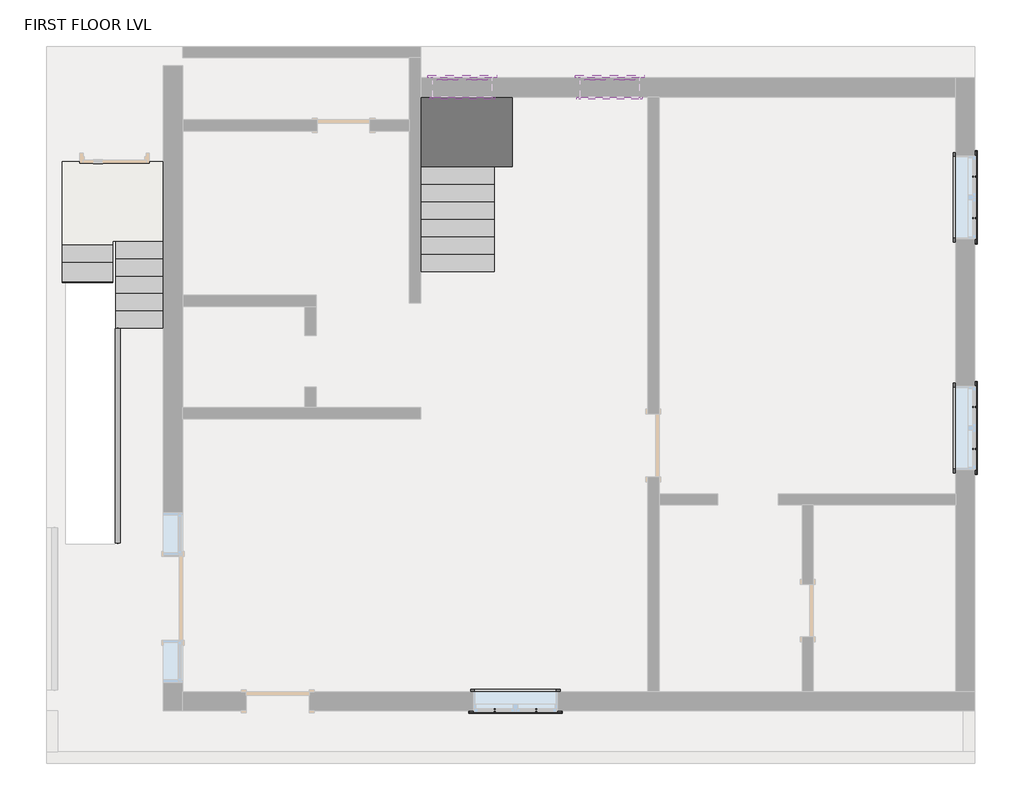
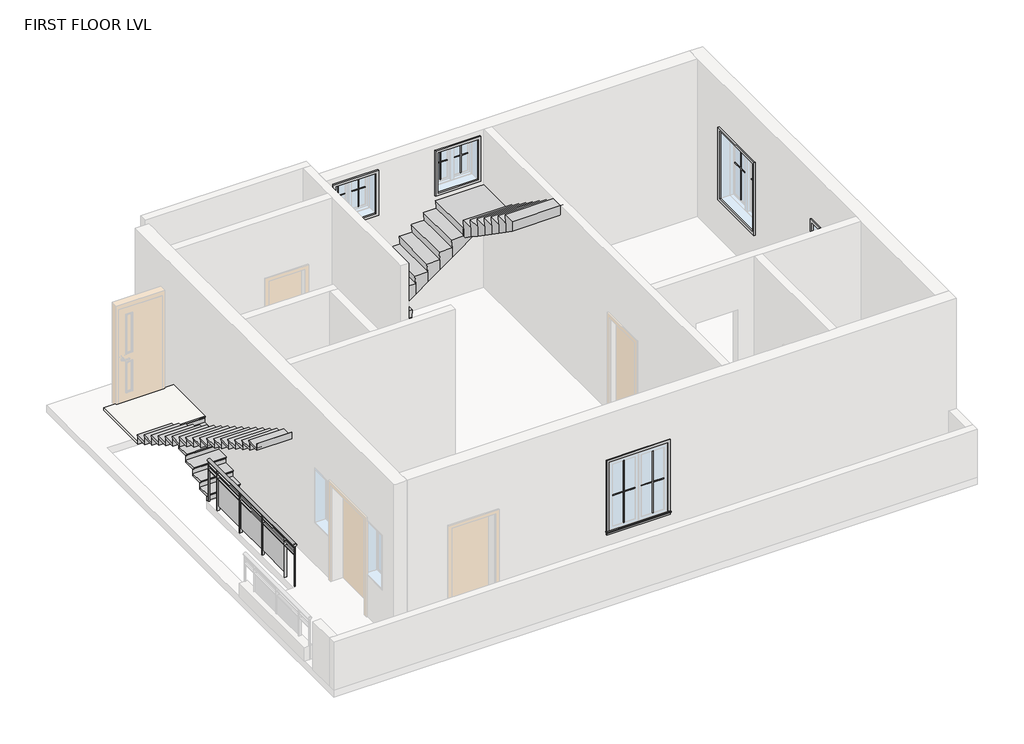
# One storey, part 2 of 2: 20 proxies, 3 stair flights, 1 railing, 1 slab.
"""IFC4 building model written with IfcOpenShell, lengths in millimetres."""

from ifc_helpers import new_model, si_unit, point, frame, origin, place, context, project, spatial, polyline, ellipse_curve, trimmed, outline, extrude, faceted_brep, transform, mapped, element, save
from ifc_brep_helpers import plane_surface, extruded_surface, advanced_brep
from components import muntin_pattern_2x2_muntin_pattern_2x2_6dad3731, muntin_pattern_2x2_muntin_pattern_2x2_a30a3345, muntin_pattern_2x2_muntin_pattern_2x2_b3fe6957, muntin_pattern_2x2_muntin_pattern_2x2_3e0ecaf2, trim_window_exterior_flat_with_sill_92b9b949, trim_window_exterior_flat_with_sill_41619996, trim_window_interior_flat_picture_frame_3bb882cf, trim_window_interior_flat_picture_frame_51c85655, non_monolithic_landing_99838e1e, stair_flight_5ae95f2f, stair_flight_f2b89c93

model = new_model("IFC4")

# Units and contexts
model_context = context("Model", 3, world=origin())
ifc_project = project(units=[si_unit("LENGTHUNIT", "METRE", prefix="MILLI")], contexts=[model_context])

# Site, building, storey
site = spatial("IfcSite", under=ifc_project)
building = spatial("IfcBuilding", under=site)
storey = spatial("IfcBuildingStorey", under=building, Name="FIRST FLOOR LVL", Elevation=3505.2)

# Proxies
placement = place(None, origin())
muntin_pattern_2x2_muntin_pattern_2x2_shape = muntin_pattern_2x2_muntin_pattern_2x2_6dad3731(model_context)
element("IfcBuildingElementProxy", 1, Name="Muntin Pattern_2x2 : Muntin Pattern_2x2", ObjectType="Muntin Pattern_2x2 : Muntin Pattern_2x2", at=placement, inside=storey, context=model_context, shape_type="MappedRepresentation", body=[
    mapped(muntin_pattern_2x2_muntin_pattern_2x2_shape, transform((46.3469404, -752.1673147, 4489.45), x_axis=(-1.0, 0.0, 0.0), y_axis=(0.0, -1.0, 0.0), z_axis=(0.0, 0.0, 1.0))),
])
element("IfcBuildingElementProxy", 2, Name="Muntin Pattern_2x2 : Muntin Pattern_2x2", ObjectType="Muntin Pattern_2x2 : Muntin Pattern_2x2", at=placement, inside=storey, context=model_context, shape_type="MappedRepresentation", body=[
    mapped(muntin_pattern_2x2_muntin_pattern_2x2_shape, transform((6420.1594404, 3662.6701853, 4489.45), x_axis=(0.0, -1.0, 0.0), y_axis=(1.0, 0.0, 0.0), z_axis=(0.0, 0.0, 1.0))),
])
element("IfcBuildingElementProxy", 3, Name="Muntin Pattern_2x2 : Muntin Pattern_2x2", ObjectType="Muntin Pattern_2x2 : Muntin Pattern_2x2", at=placement, inside=storey, context=model_context, shape_type="MappedRepresentation", body=[
    mapped(muntin_pattern_2x2_muntin_pattern_2x2_shape, transform((6420.1594404, 7021.8201853, 4489.45), x_axis=(0.0, -1.0, 0.0), y_axis=(1.0, 0.0, 0.0), z_axis=(0.0, 0.0, 1.0))),
])
muntin_pattern_2x2_muntin_pattern_2x2_2_shape = muntin_pattern_2x2_muntin_pattern_2x2_a30a3345(model_context)
element("IfcBuildingElementProxy", 4, Name="Muntin Pattern_2x2 : Muntin Pattern_2x2", ObjectType="Muntin Pattern_2x2 : Muntin Pattern_2x2", at=placement, inside=storey, context=model_context, shape_type="MappedRepresentation", body=[
    mapped(muntin_pattern_2x2_muntin_pattern_2x2_2_shape, transform((-560.0780596, -752.1673147, 4489.45), x_axis=(1.0, 0.0, 0.0), y_axis=(0.0, 1.0, 0.0), z_axis=(0.0, 0.0, 1.0))),
])
element("IfcBuildingElementProxy", 5, Name="Muntin Pattern_2x2 : Muntin Pattern_2x2", ObjectType="Muntin Pattern_2x2 : Muntin Pattern_2x2", at=placement, inside=storey, context=model_context, shape_type="MappedRepresentation", body=[
    mapped(muntin_pattern_2x2_muntin_pattern_2x2_2_shape, transform((6420.1594404, 3056.2451853, 4489.45), x_axis=(0.0, 1.0, 0.0), y_axis=(-1.0, 0.0, 0.0), z_axis=(0.0, 0.0, 1.0))),
])
element("IfcBuildingElementProxy", 6, Name="Muntin Pattern_2x2 : Muntin Pattern_2x2", ObjectType="Muntin Pattern_2x2 : Muntin Pattern_2x2", at=placement, inside=storey, context=model_context, shape_type="MappedRepresentation", body=[
    mapped(muntin_pattern_2x2_muntin_pattern_2x2_2_shape, transform((6420.1594404, 6415.3951853, 4489.45), x_axis=(0.0, 1.0, 0.0), y_axis=(-1.0, 0.0, 0.0), z_axis=(0.0, 0.0, 1.0))),
])
muntin_pattern_2x2_muntin_pattern_2x2_3_shape = muntin_pattern_2x2_muntin_pattern_2x2_b3fe6957(model_context)
element("IfcBuildingElementProxy", 7, Name="Muntin Pattern_2x2 : Muntin Pattern_2x2", ObjectType="Muntin Pattern_2x2 : Muntin Pattern_2x2", at=placement, inside=storey, context=model_context, shape_type="MappedRepresentation", body=[
    mapped(muntin_pattern_2x2_muntin_pattern_2x2_3_shape, transform((-1245.8780596, 8448.9826853, 6013.45), x_axis=(1.0, 0.0, 0.0), y_axis=(0.0, 1.0, 0.0), z_axis=(0.0, 0.0, 1.0))),
])
element("IfcBuildingElementProxy", 8, Name="Muntin Pattern_2x2 : Muntin Pattern_2x2", ObjectType="Muntin Pattern_2x2 : Muntin Pattern_2x2", at=placement, inside=storey, context=model_context, shape_type="MappedRepresentation", body=[
    mapped(muntin_pattern_2x2_muntin_pattern_2x2_3_shape, transform((900.4219404, 8448.9826853, 6013.45), x_axis=(1.0, 0.0, 0.0), y_axis=(0.0, 1.0, 0.0), z_axis=(0.0, 0.0, 1.0))),
])
muntin_pattern_2x2_muntin_pattern_2x2_4_shape = muntin_pattern_2x2_muntin_pattern_2x2_3e0ecaf2(model_context)
element("IfcBuildingElementProxy", 9, Name="Muntin Pattern_2x2 : Muntin Pattern_2x2", ObjectType="Muntin Pattern_2x2 : Muntin Pattern_2x2", at=placement, inside=storey, context=model_context, shape_type="MappedRepresentation", body=[
    mapped(muntin_pattern_2x2_muntin_pattern_2x2_4_shape, transform((-817.2530596, 8448.9826853, 6013.45), x_axis=(-1.0, 0.0, 0.0), y_axis=(0.0, -1.0, 0.0), z_axis=(0.0, 0.0, 1.0))),
])
element("IfcBuildingElementProxy", 10, Name="Muntin Pattern_2x2 : Muntin Pattern_2x2", ObjectType="Muntin Pattern_2x2 : Muntin Pattern_2x2", at=placement, inside=storey, context=model_context, shape_type="MappedRepresentation", body=[
    mapped(muntin_pattern_2x2_muntin_pattern_2x2_4_shape, transform((1329.0469404, 8448.9826853, 6013.45), x_axis=(-1.0, 0.0, 0.0), y_axis=(0.0, -1.0, 0.0), z_axis=(0.0, 0.0, 1.0))),
])
trim_window_exterior_flat_with_sill_shape = trim_window_exterior_flat_with_sill_92b9b949(model_context)
element("IfcBuildingElementProxy", 11, Name="Trim-Window-Exterior-Flat : with Sill", ObjectType="Trim-Window-Exterior-Flat : with Sill", at=placement, inside=storey, context=model_context, shape_type="MappedRepresentation", body=[
    mapped(trim_window_exterior_flat_with_sill_shape, transform((-256.8655596, -761.6923147, 5943.6), x_axis=(1.0, 0.0, 0.0), y_axis=(0.0, 0.0, 1.0), z_axis=(0.0, -1.0, 0.0))),
])
element("IfcBuildingElementProxy", 12, Name="Trim-Window-Exterior-Flat : with Sill", ObjectType="Trim-Window-Exterior-Flat : with Sill", at=placement, inside=storey, context=model_context, shape_type="MappedRepresentation", body=[
    mapped(trim_window_exterior_flat_with_sill_shape, transform((6429.6844404, 3359.4576853, 5943.6), x_axis=(0.0, 1.0, 0.0), y_axis=(0.0, 0.0, 1.0), z_axis=(1.0, 0.0, 0.0))),
])
element("IfcBuildingElementProxy", 13, Name="Trim-Window-Exterior-Flat : with Sill", ObjectType="Trim-Window-Exterior-Flat : with Sill", at=placement, inside=storey, context=model_context, shape_type="MappedRepresentation", body=[
    mapped(trim_window_exterior_flat_with_sill_shape, transform((6429.6844404, 6718.6076853, 5943.6), x_axis=(0.0, 1.0, 0.0), y_axis=(0.0, 0.0, 1.0), z_axis=(1.0, 0.0, 0.0))),
])
trim_window_exterior_flat_with_sill_2_shape = trim_window_exterior_flat_with_sill_41619996(model_context)
element("IfcBuildingElementProxy", 14, Name="Trim-Window-Exterior-Flat : with Sill", ObjectType="Trim-Window-Exterior-Flat : with Sill", at=placement, inside=storey, context=model_context, shape_type="MappedRepresentation", body=[
    mapped(trim_window_exterior_flat_with_sill_2_shape, transform((-1031.5655596, 8458.5076853, 6858.0), x_axis=(-1.0, 0.0, 0.0), y_axis=(0.0, 0.0, 1.0), z_axis=(0.0, 1.0, 0.0))),
])
element("IfcBuildingElementProxy", 15, Name="Trim-Window-Exterior-Flat : with Sill", ObjectType="Trim-Window-Exterior-Flat : with Sill", at=placement, inside=storey, context=model_context, shape_type="MappedRepresentation", body=[
    mapped(trim_window_exterior_flat_with_sill_2_shape, transform((1114.7344404, 8458.5076853, 6858.0), x_axis=(-1.0, 0.0, 0.0), y_axis=(0.0, 0.0, 1.0), z_axis=(0.0, 1.0, 0.0))),
])
trim_window_interior_flat_picture_frame_shape = trim_window_interior_flat_picture_frame_3bb882cf(model_context)
element("IfcBuildingElementProxy", 16, Name="Trim-Window-Interior-Flat : Picture Frame", ObjectType="Trim-Window-Interior-Flat : Picture Frame", at=placement, inside=storey, context=model_context, shape_type="MappedRepresentation", body=[
    mapped(trim_window_interior_flat_picture_frame_shape, transform((-256.8655596, -482.2923147, 5943.6), x_axis=(-1.0, 0.0, 0.0), y_axis=(0.0, 0.0, 1.0), z_axis=(0.0, 1.0, 0.0))),
])
element("IfcBuildingElementProxy", 17, Name="Trim-Window-Interior-Flat : Picture Frame", ObjectType="Trim-Window-Interior-Flat : Picture Frame", at=placement, inside=storey, context=model_context, shape_type="MappedRepresentation", body=[
    mapped(trim_window_interior_flat_picture_frame_shape, transform((6150.2844404, 3359.4576853, 5943.6), x_axis=(0.0, -1.0, 0.0), y_axis=(0.0, 0.0, 1.0), z_axis=(-1.0, 0.0, 0.0))),
])
element("IfcBuildingElementProxy", 18, Name="Trim-Window-Interior-Flat : Picture Frame", ObjectType="Trim-Window-Interior-Flat : Picture Frame", at=placement, inside=storey, context=model_context, shape_type="MappedRepresentation", body=[
    mapped(trim_window_interior_flat_picture_frame_shape, transform((6150.2844404, 6718.6076853, 5943.6), x_axis=(0.0, -1.0, 0.0), y_axis=(0.0, 0.0, 1.0), z_axis=(-1.0, 0.0, 0.0))),
])
trim_window_interior_flat_picture_frame_2_shape = trim_window_interior_flat_picture_frame_51c85655(model_context)
element("IfcBuildingElementProxy", 19, Name="Trim-Window-Interior-Flat : Picture Frame", ObjectType="Trim-Window-Interior-Flat : Picture Frame", at=placement, inside=storey, context=model_context, shape_type="MappedRepresentation", body=[
    mapped(trim_window_interior_flat_picture_frame_2_shape, transform((-1031.5655596, 8179.1076853, 6858.0), x_axis=(1.0, 0.0, 0.0), y_axis=(0.0, 0.0, 1.0), z_axis=(0.0, -1.0, 0.0))),
])
element("IfcBuildingElementProxy", 20, Name="Trim-Window-Interior-Flat : Picture Frame", ObjectType="Trim-Window-Interior-Flat : Picture Frame", at=placement, inside=storey, context=model_context, shape_type="MappedRepresentation", body=[
    mapped(trim_window_interior_flat_picture_frame_2_shape, transform((1114.7344404, 8179.1076853, 6858.0), x_axis=(1.0, 0.0, 0.0), y_axis=(0.0, 0.0, 1.0), z_axis=(0.0, -1.0, 0.0))),
])

# Railing
element("IfcRailing", 21, ObjectType="Glass Panel - Bottom Fill", at=placement, inside=storey, context=model_context, shape_type="SolidModel", body=[
    advanced_brep(
    [(-6008.6955596, 4807.2576853, 4419.6), (-6084.8955596, 4807.2576853, 4419.6), (-6008.6955596, 1683.0576853, 4419.6), (-6084.8955596, 1683.0576853, 4419.6)],
    [
        (0, 1, ellipse_curve(frame((-6046.7955596, 4807.2576853, 4419.6), z_axis=(0.0, 1.0, 0.0), x_axis=(-1.0, 0.0, 0.0)), 38.1, 28.575)),
        (1, 0, ellipse_curve(frame((-6046.7955596, 4807.2576853, 4419.6), z_axis=(0.0, 1.0, 0.0), x_axis=(-1.0, 0.0, 0.0)), 38.1, 28.575)),
        (2, 3, ellipse_curve(frame((-6046.7955596, 1683.0576853, 4419.6), z_axis=(0.0, -1.0, 0.0), x_axis=(-1.0, 0.0, 0.0)), 38.1, 28.575)),
        (3, 2, ellipse_curve(frame((-6046.7955596, 1683.0576853, 4419.6), z_axis=(0.0, -1.0, 0.0), x_axis=(-1.0, 0.0, 0.0)), 38.1, 28.575)),
        (0, 2),
        (3, 1),
    ],
    [
        plane_surface(frame((-6046.7955596, 4807.2576853, 4419.6), z_axis=(0.0, 1.0, 0.0), x_axis=(0.0, 0.0, -1.0))),
        plane_surface(frame((-6046.7955596, 1683.0576853, 4419.6), z_axis=(0.0, -1.0, 0.0), x_axis=(0.0, 0.0, -1.0))),
        extruded_surface(trimmed(ellipse_curve(frame((-6046.7955596, 1683.0576853, 4419.6), z_axis=(0.0, 1.0, 0.0), x_axis=(-1.0, 0.0, 0.0)), 38.1, 28.575), [point((-6008.6955596, 1683.0576853, 4419.6))], [point((-6084.8955596, 1683.0576853, 4419.6))], True, "CARTESIAN"), (0.0, 3124.2, 0.0), 3124.2),
        extruded_surface(trimmed(ellipse_curve(frame((-6046.7955596, 1683.0576853, 4419.6), z_axis=(0.0, 1.0, 0.0), x_axis=(-1.0, 0.0, 0.0)), 38.1, 28.575), [point((-6084.8955596, 1683.0576853, 4419.6))], [point((-6008.6955596, 1683.0576853, 4419.6))], True, "CARTESIAN"), (0.0, 3124.2, 0.0), 3124.2),
    ],
    [
        (0, [[1, 2]]),
        (1, [[3, 4]]),
        (2, [[-1, 5, -4, 6]]),
        (3, [[-2, -6, -3, -5]]),
    ],
),
    extrude(outline(polyline([(-6059.4955596, 4807.2576853), (-6034.0955596, 4807.2576853), (-6034.0955596, 1683.0576853), (-6059.4955596, 1683.0576853), (-6059.4955596, 4807.2576853)])), frame((0.0, 0.0, 4305.3), z_axis=(0.0, 0.0, 1.0), x_axis=(1.0, 0.0, 0.0)), (0.0, 0.0, 1.0), 25.4),
    extrude(outline(polyline([(-6059.4955596, 4807.2576853), (-6034.0955596, 4807.2576853), (-6034.0955596, 1683.0576853), (-6059.4955596, 1683.0576853), (-6059.4955596, 4807.2576853)])), frame((0.0, 0.0, 4203.7), z_axis=(0.0, 0.0, 1.0), x_axis=(1.0, 0.0, 0.0)), (0.0, 0.0, 1.0), 25.4),
    extrude(outline(polyline([(-6072.1955596, 2032.3076853), (-6021.3955596, 2032.3076853), (-6021.3955596, 2019.6076853), (-6072.1955596, 2019.6076853), (-6072.1955596, 2032.3076853)])), frame((0.0, 0.0, 3505.2), z_axis=(0.0, 0.0, 1.0), x_axis=(1.0, 0.0, 0.0)), (0.0, 0.0, 1.0), 885.825),
    extrude(outline(polyline([(-6040.2604026, 2838.7576853), (-6040.2604026, 2025.9576853), (-6046.6104026, 2025.9576853), (-6046.6104026, 2838.7576853), (-6040.2604026, 2838.7576853)])), frame((0.0, 0.0, 3606.8), z_axis=(0.0, 0.0, 1.0), x_axis=(1.0, 0.0, 0.0)), (0.0, 0.0, 1.0), 596.9),
    extrude(outline(polyline([(-6072.1955596, 2845.1076853), (-6021.3955596, 2845.1076853), (-6021.3955596, 2832.4076853), (-6072.1955596, 2832.4076853), (-6072.1955596, 2845.1076853)])), frame((0.0, 0.0, 3505.2), z_axis=(0.0, 0.0, 1.0), x_axis=(1.0, 0.0, 0.0)), (0.0, 0.0, 1.0), 885.825),
    extrude(outline(polyline([(-6040.2604026, 3651.5576853), (-6040.2604026, 2838.7576853), (-6046.6104026, 2838.7576853), (-6046.6104026, 3651.5576853), (-6040.2604026, 3651.5576853)])), frame((0.0, 0.0, 3606.8), z_axis=(0.0, 0.0, 1.0), x_axis=(1.0, 0.0, 0.0)), (0.0, 0.0, 1.0), 596.9),
    extrude(outline(polyline([(-6072.1955596, 3657.9076853), (-6021.3955596, 3657.9076853), (-6021.3955596, 3645.2076853), (-6072.1955596, 3645.2076853), (-6072.1955596, 3657.9076853)])), frame((0.0, 0.0, 3505.2), z_axis=(0.0, 0.0, 1.0), x_axis=(1.0, 0.0, 0.0)), (0.0, 0.0, 1.0), 885.825),
    extrude(outline(polyline([(-6040.2604026, 4464.3576853), (-6040.2604026, 3651.5576853), (-6046.6104026, 3651.5576853), (-6046.6104026, 4464.3576853), (-6040.2604026, 4464.3576853)])), frame((0.0, 0.0, 3606.8), z_axis=(0.0, 0.0, 1.0), x_axis=(1.0, 0.0, 0.0)), (0.0, 0.0, 1.0), 596.9),
    extrude(outline(polyline([(-6072.1955596, 4470.7076853), (-6021.3955596, 4470.7076853), (-6021.3955596, 4458.0076853), (-6072.1955596, 4458.0076853), (-6072.1955596, 4470.7076853)])), frame((0.0, 0.0, 3505.2), z_axis=(0.0, 0.0, 1.0), x_axis=(1.0, 0.0, 0.0)), (0.0, 0.0, 1.0), 885.825),
    extrude(outline(polyline([(-6056.3205596, 1695.7576853), (-6037.2705596, 1695.7576853), (-6037.2705596, 1676.7076853), (-6056.3205596, 1676.7076853), (-6056.3205596, 1695.7576853)])), frame((0.0, 0.0, 3505.2), z_axis=(0.0, 0.0, 1.0), x_axis=(1.0, 0.0, 0.0)), (0.0, 0.0, 1.0), 885.825),
    extrude(outline(polyline([(-6056.3205596, 4813.6076853), (-6037.2705596, 4813.6076853), (-6037.2705596, 4794.5576853), (-6056.3205596, 4794.5576853), (-6056.3205596, 4813.6076853)])), frame((0.0, 0.0, 3505.2), z_axis=(0.0, 0.0, 1.0), x_axis=(1.0, 0.0, 0.0)), (0.0, 0.0, 1.0), 885.825),
])

# Slab
non_monolithic_landing_shape = non_monolithic_landing_99838e1e(model_context)
element("IfcSlab", 22, ObjectType="Non-Monolithic Landing", at=placement, inside=storey, context=model_context, shape_type="MappedRepresentation", body=[
    mapped(non_monolithic_landing_shape, transform((0.0, 0.0, 0.0), x_axis=(1.0, 0.0, 0.0), y_axis=(0.0, 1.0, 0.0), z_axis=(0.0, 0.0, 1.0))),
])

# Stair flights
stair_flight_shape = stair_flight_5ae95f2f(model_context)
element("IfcStairFlight", 23, ObjectType="2\" Tread 1\" Nosing 1/4\" Riser", at=placement, inside=storey, context=model_context, shape_type="MappedRepresentation", body=[
    mapped(stair_flight_shape, transform((0.0, 0.0, 0.0), x_axis=(1.0, 0.0, 0.0), y_axis=(0.0, 1.0, 0.0), z_axis=(0.0, 0.0, 1.0))),
])
stair_flight_2_shape = stair_flight_f2b89c93(model_context)
element("IfcStairFlight", 24, ObjectType="2\" Tread 1\" Nosing 1/4\" Riser", at=placement, inside=storey, context=model_context, shape_type="MappedRepresentation", body=[
    mapped(stair_flight_2_shape, transform((0.0, 0.0, 0.0), x_axis=(1.0, 0.0, 0.0), y_axis=(0.0, 1.0, 0.0), z_axis=(0.0, 0.0, 1.0))),
])
element("IfcStairFlight", 25, ObjectType="3/4\" Nosing 6 1/2\" Depth", at=placement, inside=storey, context=model_context, shape_type="Brep", body=[
    faceted_brep([(-568.0155596, 5639.1076853, 3680.46), (-1634.8155596, 5639.1076853, 3680.46), (-1634.8155596, 5658.1576853, 3505.2), (-568.0155596, 5658.1576853, 3505.2), (-568.0155596, 5912.1576853, 3680.46), (-1634.8155596, 5912.1576853, 3680.46), (-1634.8155596, 5912.1576853, 3505.2), (-568.0155596, 5912.1576853, 3505.2), (-1634.8155596, 5893.1076853, 3855.72), (-568.0155596, 5893.1076853, 3855.72), (-568.0155596, 6166.1576853, 3855.72), (-1634.8155596, 6166.1576853, 3855.72), (-1634.8155596, 6166.1576853, 3655.131993), (-1634.8155596, 5948.8649419, 3505.2), (-568.0155596, 5948.8649419, 3505.2), (-568.0155596, 6166.1576853, 3655.131993), (-1634.8155596, 6147.1076853, 4030.98), (-568.0155596, 6147.1076853, 4030.98), (-568.0155596, 6420.1576853, 4030.98), (-1634.8155596, 6420.1576853, 4030.98), (-1634.8155596, 6420.1576853, 3830.391993), (-568.0155596, 6420.1576853, 3830.391993), (-1634.8155596, 6401.1076853, 4206.24), (-568.0155596, 6401.1076853, 4206.24), (-568.0155596, 6674.1576853, 4206.24), (-1634.8155596, 6674.1576853, 4206.24), (-1634.8155596, 6674.1576853, 4005.651993), (-568.0155596, 6674.1576853, 4005.651993), (-1634.8155596, 6655.1076853, 4381.5), (-568.0155596, 6655.1076853, 4381.5), (-568.0155596, 6928.1576853, 4381.5), (-1634.8155596, 6928.1576853, 4381.5), (-1634.8155596, 6928.1576853, 4180.911993), (-568.0155596, 6928.1576853, 4180.911993), (-1634.8155596, 6909.1076853, 4556.76), (-568.0155596, 6909.1076853, 4556.76), (-568.0155596, 7182.1576853, 4556.76), (-1634.8155596, 7182.1576853, 4556.76), (-1634.8155596, 7182.1576853, 4356.171993), (-568.0155596, 7487.5895795, 4566.92), (-568.0155596, 7181.0533375, 4566.92), (-548.9655596, 8229.9076853, 4732.02), (-1634.8155596, 8229.9076853, 4732.02), (-1634.8155596, 7487.5895795, 4732.02), (-1634.8155596, 7163.1076853, 4732.02), (-568.0155596, 7163.1076853, 4732.02), (-548.9655596, 7163.1076853, 4732.02), (-548.9655596, 8229.9076853, 4566.92), (-1634.8155596, 8229.9076853, 4566.92), (-1634.8155596, 7487.5895795, 4566.92), (-568.0155596, 7163.1076853, 4566.92), (-548.9655596, 7163.1076853, 4566.92), (-568.0155596, 8229.9076853, 4907.28), (-568.0155596, 7163.1076853, 4907.28), (-495.7881346, 7163.1076853, 4907.28), (-345.7655596, 7163.1076853, 4907.28), (-345.7655596, 8229.9076853, 4907.28), (-495.7881346, 8229.9076853, 4907.28), (-345.7655596, 8229.9076853, 4674.7487258), (-495.7881346, 8229.9076853, 4566.92), (-495.7881346, 7163.1076853, 4566.92), (-345.7655596, 7163.1076853, 4674.7487258), (-364.8155596, 8229.9076853, 5082.54), (-364.8155596, 7163.1076853, 5082.54), (-91.7655596, 7163.1076853, 5082.54), (-91.7655596, 8229.9076853, 5082.54), (-91.7655596, 8229.9076853, 4857.3112258), (-91.7655596, 7163.1076853, 4857.3112258), (-110.8155596, 8229.9076853, 5257.8), (-110.8155596, 7163.1076853, 5257.8), (162.2344404, 7163.1076853, 5257.8), (162.2344404, 8229.9076853, 5257.8), (162.2344404, 8229.9076853, 5039.8737258), (162.2344404, 7163.1076853, 5039.8737258), (143.1844404, 8229.9076853, 5433.06), (143.1844404, 7163.1076853, 5433.06), (416.2344404, 7163.1076853, 5433.06), (416.2344404, 8229.9076853, 5433.06), (416.2344404, 8229.9076853, 5222.4362258), (416.2344404, 7163.1076853, 5222.4362258), (397.1844404, 8229.9076853, 5608.32), (397.1844404, 7163.1076853, 5608.32), (670.2344404, 7163.1076853, 5608.32), (670.2344404, 8229.9076853, 5608.32), (670.2344404, 8229.9076853, 5404.9987258), (967.2518654, 7163.1076853, 5618.48), (669.1300926, 7163.1076853, 5618.48), (1717.9844404, 7144.0576853, 5783.58), (1717.9844404, 8229.9076853, 5783.58), (967.2518654, 8229.9076853, 5783.58), (651.1844404, 8229.9076853, 5783.58), (651.1844404, 7163.1076853, 5783.58), (651.1844404, 7144.0576853, 5783.58), (1717.9844404, 7144.0576853, 5618.48), (1717.9844404, 8229.9076853, 5618.48), (967.2518654, 8229.9076853, 5618.48), (651.1844404, 7163.1076853, 5618.48), (651.1844404, 7144.0576853, 5618.48), (1717.9844404, 7163.1076853, 5958.84), (651.1844404, 7163.1076853, 5958.84), (651.1844404, 7092.6257911, 5958.84), (651.1844404, 6890.0576853, 5958.84), (1717.9844404, 6890.0576853, 5958.84), (1717.9844404, 7092.6257911, 5958.84), (1717.9844404, 6890.0576853, 5758.251993), (1717.9844404, 7092.6257911, 5618.48), (651.1844404, 7092.6257911, 5618.48), (651.1844404, 6890.0576853, 5758.251993), (1717.9844404, 6909.1076853, 6134.1), (651.1844404, 6909.1076853, 6134.1), (651.1844404, 6636.0576853, 6134.1), (1717.9844404, 6636.0576853, 6134.1), (1717.9844404, 6636.0576853, 5933.511993), (651.1844404, 6636.0576853, 5933.511993), (1717.9844404, 6655.1076853, 6309.36), (651.1844404, 6655.1076853, 6309.36), (651.1844404, 6382.0576853, 6309.36), (1717.9844404, 6382.0576853, 6309.36), (1717.9844404, 6382.0576853, 6108.771993), (651.1844404, 6382.0576853, 6108.771993), (1717.9844404, 6401.1076853, 6484.62), (651.1844404, 6401.1076853, 6484.62), (651.1844404, 6128.0576853, 6484.62), (1717.9844404, 6128.0576853, 6484.62), (1717.9844404, 6128.0576853, 6284.031993), (651.1844404, 6128.0576853, 6284.031993), (1717.9844404, 6147.1076853, 6659.88), (651.1844404, 6147.1076853, 6659.88), (651.1844404, 5874.0576853, 6659.88), (1717.9844404, 5874.0576853, 6659.88), (1717.9844404, 5874.0576853, 6459.291993), (651.1844404, 5874.0576853, 6459.291993), (1717.9844404, 5893.1076853, 6835.14), (651.1844404, 5893.1076853, 6835.14), (651.1844404, 5620.0576853, 6835.14), (1717.9844404, 5620.0576853, 6835.14), (1717.9844404, 5620.0576853, 6634.551993), (651.1844404, 5620.0576853, 6634.551993), (1717.9844404, 5639.1076853, 7010.4), (651.1844404, 5639.1076853, 7010.4), (651.1844404, 5385.1076853, 7010.4), (1717.9844404, 5385.1076853, 7010.4), (1717.9844404, 5385.1076853, 6796.667493), (651.1844404, 5385.1076853, 6796.667493)], [[[0, 1, 2, 3]], [[1, 0, 4, 5]], [[1, 5, 6, 2]], [[4, 0, 3, 7]], [[8, 9, 10, 11]], [[6, 5, 8, 11, 12, 13]], [[4, 7, 14, 15, 10, 9]], [[5, 4, 9, 8]], [[16, 17, 18, 19]], [[16, 19, 20, 12, 11]], [[18, 17, 10, 15, 21]], [[11, 10, 17, 16]], [[22, 23, 24, 25]], [[22, 25, 26, 20, 19]], [[24, 23, 18, 21, 27]], [[19, 18, 23, 22]], [[28, 29, 30, 31]], [[28, 31, 32, 26, 25]], [[30, 29, 24, 27, 33]], [[25, 24, 29, 28]], [[34, 35, 36, 37]], [[34, 37, 38, 32, 31]], [[35, 30, 33, 39, 40, 36]], [[31, 30, 35, 34]], [[41, 42, 43, 44, 45, 46]], [[42, 41, 47, 48]], [[37, 44, 43, 42, 48, 49, 38]], [[45, 40, 50]], [[46, 45, 50, 51]], [[37, 36, 40, 45, 44]], [[52, 53, 54, 55, 56, 57]], [[41, 52, 57, 56, 58, 59, 47]], [[53, 46, 51, 60, 61, 55, 54]], [[41, 46, 53, 52]], [[62, 63, 64, 65]], [[62, 65, 66, 58, 56]], [[64, 63, 55, 61, 67]], [[56, 55, 63, 62]], [[68, 69, 70, 71]], [[68, 71, 72, 66, 65]], [[70, 69, 64, 67, 73]], [[65, 64, 69, 68]], [[74, 75, 76, 77]], [[74, 77, 78, 72, 71]], [[76, 75, 70, 73, 79]], [[71, 70, 75, 74]], [[80, 81, 82, 83]], [[80, 83, 84, 78, 77]], [[81, 76, 79, 85, 86, 82]], [[77, 76, 81, 80]], [[87, 88, 89, 90, 91, 92]], [[88, 87, 93, 94]], [[83, 90, 89, 88, 94, 95, 84]], [[91, 86, 96]], [[92, 91, 96, 97]], [[83, 82, 86, 91, 90]], [[98, 99, 100, 101, 102, 103]], [[87, 98, 103, 102, 104, 105, 93]], [[99, 92, 97, 106, 107, 101, 100]], [[87, 92, 99, 98]], [[108, 109, 110, 111]], [[108, 111, 112, 104, 102]], [[110, 109, 101, 107, 113]], [[102, 101, 109, 108]], [[114, 115, 116, 117]], [[114, 117, 118, 112, 111]], [[116, 115, 110, 113, 119]], [[111, 110, 115, 114]], [[120, 121, 122, 123]], [[120, 123, 124, 118, 117]], [[122, 121, 116, 119, 125]], [[117, 116, 121, 120]], [[126, 127, 128, 129]], [[126, 129, 130, 124, 123]], [[128, 127, 122, 125, 131]], [[123, 122, 127, 126]], [[132, 133, 134, 135]], [[132, 135, 136, 130, 129]], [[134, 133, 128, 131, 137]], [[129, 128, 133, 132]], [[138, 139, 140, 141]], [[138, 141, 142, 136, 135]], [[140, 139, 134, 137, 143]], [[141, 140, 143, 142]], [[135, 134, 139, 138]], [[2, 6, 13, 14, 7, 3]], [[49, 39, 33, 27, 21, 15, 14, 13, 12, 20, 26, 32, 38]], [[39, 49, 48, 47, 59, 60, 51, 50, 40]], [[60, 59, 58, 66, 72, 78, 84, 95, 85, 79, 73, 67, 61]], [[85, 95, 94, 93, 105, 106, 97, 96, 86]], [[106, 105, 104, 112, 118, 124, 130, 136, 142, 143, 137, 131, 125, 119, 113, 107]]]),
])

save(model, "model.ifc")

# Revit data of these elements
# Type "Muntin Pattern_2x2 : Muntin Pattern_2x2"
#   Width [instance default] = 4' - 0"
#   Thickness = 0' - 0 1/2"
#   Height [instance default] = 4' - 0"
#   Distance = 0' - 0 3/4"
#   Interior Material [instance default] = none
#   Exterior Material [instance default] = none
#   Default Elevation = 0
# Type "Trim-Window-Exterior-Flat : with Sill"
#   Trim Width = 0' - 2 1/4"
#   Trim Thickness_Picture Frame = 0' - 1 1/4"
#   Trim Thickness_with Sill = 0' - 0 3/4"
#   Sill Thickness = 0' - 1 1/4"
#   Opening Width [instance default] = 2' - 0"
#   Opening Height [instance default] = 3' - 0"
#   Default Elevation = 4' - 0"
#   Sill = yes
#   Picture Frame = no
#   Trim Material [instance default] = none
# Type "Trim-Window-Interior-Flat : Picture Frame"
#   Trim Thickness_Picture Frame = 0' - 1 1/4"
#   Trim Width = 0' - 2 1/4"
#   Trim Thickness_with Sill = 0' - 0 3/4"
#   Sill Thickness = 0' - 1 1/4"
#   Opening Width [instance default] = 2' - 0"
#   Opening Height [instance default] = 3' - 0"
#   Default Elevation = 4' - 0"
#   Sill = no
#   Picture Frame = yes
#   Trim Material [instance default] = none
# Type "Glass Panel - Bottom Fill"
#   Assembly Code = "C2010400"
#   built-in parameter 1008612 = 0.0416667 (stored number, unit not read)
#   built-in parameter 1008611 = 0.0416667 (stored number, unit not read)
#   built-in parameter 1008609 = 0.333333 (stored number, unit not read)
#   built-in parameter 1008604 = 0.166667 (stored number, unit not read)
#   built-in parameter 1008603 = 0.166667 (stored number, unit not read)
#   Railing Height = 3' - 0"
#   built-in parameter 1008630 = 2
#   built-in parameter 1008610 = 2
#   built-in parameter 1008618 = Baluster - Square : 3/4"
# Elements 1, 2, 3, 4, 5, 6 (IfcBuildingElementProxy, "Muntin Pattern_2x2 : Muntin Pattern_2x2")
#   Width = 1' - 6 5/8"
#   Height = 4' - 6 1/2"
#   Interior Material = Wood - Stained
#   Exterior Material = Clad - White
#   Phase Created = New Construction
#   Materials on its faces: "Clad - White", "Wood - Stained"
# Elements 7, 8, 9, 10 (IfcBuildingElementProxy, "Muntin Pattern_2x2 : Muntin Pattern_2x2")
#   Width = 0' - 11 5/8"
#   Height = 2' - 6 1/2"
#   Interior Material = Wood - Stained
#   Exterior Material = Clad - White
#   Phase Created = New Construction
#   Materials on its faces: "Clad - White", "Wood - Stained"
# Elements 11, 12, 13 (IfcBuildingElementProxy, "Trim-Window-Exterior-Flat : with Sill")
#   Opening Width = 4' - 0"
#   Opening Height = 5' - 0"
#   Trim Material = Clad - White
#   Phase Created = New Construction
#   Materials on its faces: "Clad - White"
# Elements 14, 15 (IfcBuildingElementProxy, "Trim-Window-Exterior-Flat : with Sill")
#   Opening Width = 2' - 10"
#   Opening Height = 3' - 0"
#   Trim Material = Clad - White
#   Phase Created = New Construction
#   Materials on its faces: "Clad - White"
# Elements 16, 17, 18 (IfcBuildingElementProxy, "Trim-Window-Interior-Flat : Picture Frame")
#   Opening Width = 4' - 0"
#   Opening Height = 5' - 0"
#   Trim Material = Wood - Stained
#   Phase Created = New Construction
#   Materials on its faces: "Wood - Stained"
# Elements 19, 20 (IfcBuildingElementProxy, "Trim-Window-Interior-Flat : Picture Frame")
#   Opening Width = 2' - 10"
#   Opening Height = 3' - 0"
#   Trim Material = Wood - Stained
#   Phase Created = New Construction
#   Materials on its faces: "Wood - Stained"
# Element 21 (IfcRailing, "Glass Panel - Bottom Fill")
#   Phase Created = New Construction
#   Materials on its faces: "Glass"
# Element 22 (IfcSlab, "Non-Monolithic Landing")
#   Phase Created = New Construction
# Elements 23, 24 (IfcStairFlight, "2\" Tread 1\" Nosing 1/4\" Riser")
#   Phase Created = New Construction
# Element 25 (IfcStairFlight, "3/4\" Nosing 6 1/2\" Depth")
#   Phase Created = New Construction
#   Materials on its faces: "Concrete, Cast-in-Place gray"
# Materials
#   "Clad - White": class "Wood", colour RGB 242 242 238, transparency 0, Cost = 0
#   "Wood - Stained": class "Wood", colour RGB 224 178 126, transparency 0, Cost = 0
#   "Glass": class "Glass", colour RGB 0 128 192, transparency 0.75, Description = "Soda Lime Glass", Cost = 0
#   "Concrete, Cast-in-Place gray": class "Concrete", colour RGB 192 192 192, transparency 0, Description = "Cast-in-place concrete", Cost = 0
